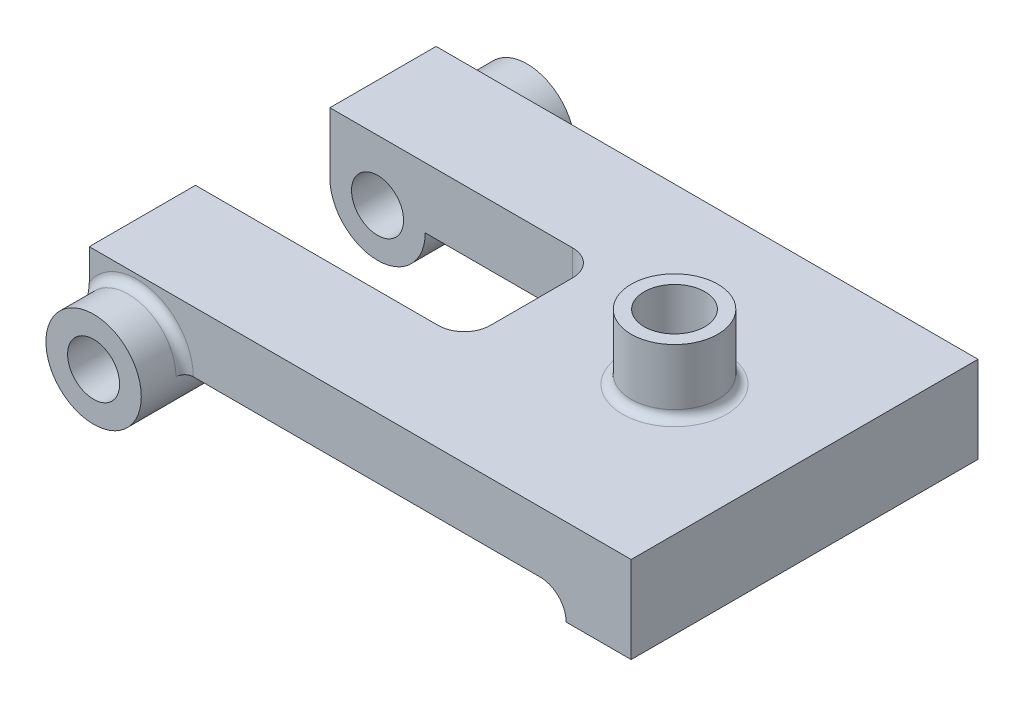
ISO-10303-21;
HEADER;
FILE_DESCRIPTION(('STEP AP214'),'2;1');
FILE_NAME('part.step','',(''),(''),'','','');
FILE_SCHEMA(('AUTOMOTIVE_DESIGN { 1 0 10303 214 1 1 1 1 }'));
ENDSEC;
DATA;
#1=APPLICATION_CONTEXT('core data for automotive mechanical design processes');
#2=APPLICATION_PROTOCOL_DEFINITION('international standard','automotive_design',2000,#1);
#3=PRODUCT_CONTEXT('',#1,'mechanical');
#4=PRODUCT('Part','Part','',(#3));
#5=PRODUCT_RELATED_PRODUCT_CATEGORY('part','',(#4));
#6=PRODUCT_DEFINITION_FORMATION('','',#4);
#7=PRODUCT_DEFINITION_CONTEXT('part definition',#1,'design');
#8=PRODUCT_DEFINITION('design','',#6,#7);
#9=PRODUCT_DEFINITION_SHAPE('','',#8);
#10=(LENGTH_UNIT() NAMED_UNIT(*) SI_UNIT(.MILLI.,.METRE.));
#11=(NAMED_UNIT(*) PLANE_ANGLE_UNIT() SI_UNIT($,.RADIAN.));
#12=(NAMED_UNIT(*) SI_UNIT($,.STERADIAN.) SOLID_ANGLE_UNIT());
#13=UNCERTAINTY_MEASURE_WITH_UNIT(LENGTH_MEASURE(1.E-05),#10,'distance_accuracy_value','');
#14=(GEOMETRIC_REPRESENTATION_CONTEXT(3) GLOBAL_UNCERTAINTY_ASSIGNED_CONTEXT((#13)) GLOBAL_UNIT_ASSIGNED_CONTEXT((#10,
#11,#12)) REPRESENTATION_CONTEXT('',''));
#15=CARTESIAN_POINT('',(0.,0.,0.));
#16=DIRECTION('',(0.,0.,1.));
#17=DIRECTION('',(1.,0.,0.));
#18=AXIS2_PLACEMENT_3D('',#15,#16,#17);
#19=CARTESIAN_POINT('',(0.,0.,40.));
#20=DIRECTION('',(-1.,0.,0.));
#21=DIRECTION('',(0.,0.,1.));
#22=AXIS2_PLACEMENT_3D('',#19,#20,#21);
#23=PLANE('',#22);
#24=DIRECTION('',(0.,1.,0.));
#25=VECTOR('',#24,1.);
#26=CARTESIAN_POINT('',(0.,-91.,15.5));
#27=LINE('',#26,#25);
#28=CARTESIAN_POINT('',(0.,0.,15.5));
#29=VERTEX_POINT('',#28);
#30=CARTESIAN_POINT('',(0.,14.,15.5));
#31=VERTEX_POINT('',#30);
#32=EDGE_CURVE('E184',#29,#31,#27,.T.);
#33=ORIENTED_EDGE('',*,*,#32,.F.);
#34=DIRECTION('',(0.,0.,-1.));
#35=VECTOR('',#34,1.);
#36=CARTESIAN_POINT('',(0.,0.,40.));
#37=LINE('',#36,#35);
#38=CARTESIAN_POINT('',(0.,0.,42.));
#39=VERTEX_POINT('',#38);
#40=EDGE_CURVE('E265',#39,#29,#37,.T.);
#41=ORIENTED_EDGE('',*,*,#40,.F.);
#42=CARTESIAN_POINT('',(0.,6.92820323027551,40.));
#43=CARTESIAN_POINT('',(0.,6.79631878338538,40.0000195877206));
#44=CARTESIAN_POINT('',(0.,6.6644773142545,40.0037039568171));
#45=CARTESIAN_POINT('',(0.,6.40121335984525,40.0176384033789));
#46=CARTESIAN_POINT('',(0.,6.26979067374991,40.0278846179913));
#47=CARTESIAN_POINT('',(0.,6.00790763005172,40.0541440086299));
#48=CARTESIAN_POINT('',(0.,5.8774456101869,40.0701410055856));
#49=CARTESIAN_POINT('',(0.,5.61724352656619,40.1072767015453));
#50=CARTESIAN_POINT('',(0.,5.48750358375657,40.1284162368858));
#51=CARTESIAN_POINT('',(0.,5.10222369832927,40.1981930126899));
#52=CARTESIAN_POINT('',(0.,4.84787990643271,40.2534888297203));
#53=CARTESIAN_POINT('',(0.,4.34256909228623,40.3782545428354));
#54=CARTESIAN_POINT('',(0.,4.09160501060128,40.4477360266855));
#55=CARTESIAN_POINT('',(0.,3.51579220612537,40.6210301613932));
#56=CARTESIAN_POINT('',(0.,3.1921467958774,40.7288093836496));
#57=CARTESIAN_POINT('',(0.,2.54957173398162,40.9576910405927));
#58=CARTESIAN_POINT('',(0.,2.23064375632872,41.0787980818546));
#59=CARTESIAN_POINT('',(0.,1.27744390124962,41.455368919855));
#60=CARTESIAN_POINT('',(0.,0.648288026431028,41.7235697880645));
#61=CARTESIAN_POINT('',(0.,0.0128635078759241,41.9945149951131));
#62=CARTESIAN_POINT('',(0.,0.00643174896304407,41.9972575065247));
#63=CARTESIAN_POINT('',(0.,0.,42.));
#64=B_SPLINE_CURVE_WITH_KNOTS('',3,(#42,#43,#44,#45,#46,#47,#48,#49,#50,#51,#52,#53,#54,#55,#56,
#57,#58,#59,#60,#61,#62,#63),.UNSPECIFIED.,.F.,.F.,(4,2,2,2,2,2,2,2,2,2,4),(0.,
0.395540642762623,0.790848650888232,1.18505310551169,1.57932171293576,2.35959856433425,
3.14051536472973,4.16341984179192,5.1866789886057,7.23803512077281,7.25901129773622),.UNSPECIFIED.);
#65=CARTESIAN_POINT('',(0.,6.92820323027551,40.));
#66=VERTEX_POINT('',#65);
#67=EDGE_CURVE('E278',#39,#66,#64,.F.);
#68=ORIENTED_EDGE('',*,*,#67,.T.);
#69=DIRECTION('',(0.,1.,0.));
#70=VECTOR('',#69,1.);
#71=CARTESIAN_POINT('',(0.,0.,40.));
#72=LINE('',#71,#70);
#73=CARTESIAN_POINT('',(0.,14.,40.));
#74=VERTEX_POINT('',#73);
#75=EDGE_CURVE('E231',#66,#74,#72,.T.);
#76=ORIENTED_EDGE('',*,*,#75,.T.);
#77=DIRECTION('',(0.,0.,-1.));
#78=VECTOR('',#77,1.);
#79=CARTESIAN_POINT('',(0.,14.,40.));
#80=LINE('',#79,#78);
#81=EDGE_CURVE('E270',#74,#31,#80,.T.);
#82=ORIENTED_EDGE('',*,*,#81,.T.);
#83=EDGE_LOOP('',(#33,#41,#68,#76,#82));
#84=FACE_BOUND('',#83,.T.);
#85=ADVANCED_FACE('F41',(#84),#23,.T.);
#86=CARTESIAN_POINT('',(11.,0.,50.));
#87=DIRECTION('',(0.,0.,-1.));
#88=DIRECTION('',(-1.,0.,0.));
#89=AXIS2_PLACEMENT_3D('',#86,#87,#88);
#90=CYLINDRICAL_SURFACE('',#89,6.);
#91=CARTESIAN_POINT('',(11.,0.,15.5));
#92=DIRECTION('',(0.,0.,1.));
#93=DIRECTION('',(1.,0.,0.));
#94=AXIS2_PLACEMENT_3D('',#91,#92,#93);
#95=CIRCLE('',#94,6.);
#96=CARTESIAN_POINT('',(5.,0.,15.5));
#97=VERTEX_POINT('',#96);
#98=EDGE_CURVE('E199',#97,#97,#95,.T.);
#99=CARTESIAN_POINT('',(11.,0.,50.));
#100=DIRECTION('',(0.,0.,1.));
#101=DIRECTION('',(1.,0.,0.));
#102=AXIS2_PLACEMENT_3D('',#99,#100,#101);
#103=CIRCLE('',#102,6.);
#104=CARTESIAN_POINT('',(5.,0.,50.));
#105=VERTEX_POINT('',#104);
#106=EDGE_CURVE('E206',#105,#105,#103,.T.);
#107=CARTESIAN_POINT('',(5.,0.,15.5));
#108=CARTESIAN_POINT('',(5.,0.,15.859375));
#109=CARTESIAN_POINT('',(5.,0.,16.21875));
#110=CARTESIAN_POINT('',(5.,0.,16.9375));
#111=CARTESIAN_POINT('',(5.,0.,17.296875));
#112=CARTESIAN_POINT('',(5.,0.,18.015625));
#113=CARTESIAN_POINT('',(5.,0.,18.375));
#114=CARTESIAN_POINT('',(5.,0.,19.09375));
#115=CARTESIAN_POINT('',(5.,0.,19.453125));
#116=CARTESIAN_POINT('',(5.,0.,20.171875));
#117=CARTESIAN_POINT('',(5.,0.,20.53125));
#118=CARTESIAN_POINT('',(5.,0.,21.25));
#119=CARTESIAN_POINT('',(5.,0.,21.609375));
#120=CARTESIAN_POINT('',(5.,0.,22.328125));
#121=CARTESIAN_POINT('',(5.,0.,22.6875));
#122=CARTESIAN_POINT('',(5.,0.,23.40625));
#123=CARTESIAN_POINT('',(5.,0.,23.765625));
#124=CARTESIAN_POINT('',(5.,0.,24.484375));
#125=CARTESIAN_POINT('',(5.,0.,24.84375));
#126=CARTESIAN_POINT('',(5.,0.,25.5625));
#127=CARTESIAN_POINT('',(5.,0.,25.921875));
#128=CARTESIAN_POINT('',(5.,0.,26.640625));
#129=CARTESIAN_POINT('',(5.,0.,27.));
#130=CARTESIAN_POINT('',(5.,0.,27.71875));
#131=CARTESIAN_POINT('',(5.,0.,28.078125));
#132=CARTESIAN_POINT('',(5.,0.,28.796875));
#133=CARTESIAN_POINT('',(5.,0.,29.15625));
#134=CARTESIAN_POINT('',(5.,0.,29.875));
#135=CARTESIAN_POINT('',(5.,0.,30.234375));
#136=CARTESIAN_POINT('',(5.,0.,30.953125));
#137=CARTESIAN_POINT('',(5.,0.,31.3125));
#138=CARTESIAN_POINT('',(5.,0.,32.03125));
#139=CARTESIAN_POINT('',(5.,0.,32.390625));
#140=CARTESIAN_POINT('',(5.,0.,33.109375));
#141=CARTESIAN_POINT('',(5.,0.,33.46875));
#142=CARTESIAN_POINT('',(5.,0.,34.1875));
#143=CARTESIAN_POINT('',(5.,0.,34.546875));
#144=CARTESIAN_POINT('',(5.,0.,35.265625));
#145=CARTESIAN_POINT('',(5.,0.,35.625));
#146=CARTESIAN_POINT('',(5.,0.,36.34375));
#147=CARTESIAN_POINT('',(5.,0.,36.703125));
#148=CARTESIAN_POINT('',(5.,0.,37.421875));
#149=CARTESIAN_POINT('',(5.,0.,37.78125));
#150=CARTESIAN_POINT('',(5.,0.,38.5));
#151=CARTESIAN_POINT('',(5.,0.,38.859375));
#152=CARTESIAN_POINT('',(5.,0.,39.578125));
#153=CARTESIAN_POINT('',(5.,0.,39.9375));
#154=CARTESIAN_POINT('',(5.,0.,40.65625));
#155=CARTESIAN_POINT('',(5.,0.,41.015625));
#156=CARTESIAN_POINT('',(5.,0.,41.734375));
#157=CARTESIAN_POINT('',(5.,0.,42.09375));
#158=CARTESIAN_POINT('',(5.,0.,42.8125));
#159=CARTESIAN_POINT('',(5.,0.,43.171875));
#160=CARTESIAN_POINT('',(5.,0.,43.890625));
#161=CARTESIAN_POINT('',(5.,0.,44.25));
#162=CARTESIAN_POINT('',(5.,0.,44.96875));
#163=CARTESIAN_POINT('',(5.,0.,45.328125));
#164=CARTESIAN_POINT('',(5.,0.,46.046875));
#165=CARTESIAN_POINT('',(5.,0.,46.40625));
#166=CARTESIAN_POINT('',(5.,0.,47.125));
#167=CARTESIAN_POINT('',(5.,0.,47.484375));
#168=CARTESIAN_POINT('',(5.,0.,48.203125));
#169=CARTESIAN_POINT('',(5.,0.,48.5625));
#170=CARTESIAN_POINT('',(5.,0.,49.28125));
#171=CARTESIAN_POINT('',(5.,0.,49.640625));
#172=CARTESIAN_POINT('',(5.,0.,50.));
#173=B_SPLINE_CURVE_WITH_KNOTS('',3,(#107,#108,#109,#110,#111,#112,#113,#114,#115,#116,#117,
#118,#119,#120,#121,#122,#123,#124,#125,#126,#127,#128,#129,#130,#131,#132,#133,#134,#135,#136,
#137,#138,#139,#140,#141,#142,#143,#144,#145,#146,#147,#148,#149,#150,#151,#152,#153,#154,#155,
#156,#157,#158,#159,#160,#161,#162,#163,#164,#165,#166,#167,#168,#169,#170,#171,#172),
.UNSPECIFIED.,.F.,.F.,(4,2,2,2,2,2,2,2,2,2,2,2,2,2,2,2,2,2,2,2,2,2,2,2,2,2,2,2,2,2,2,2,4),(0.,
1.078125,2.15625,3.234375,4.31249999999999,5.39062499999999,6.46874999999999,7.54687499999999,
8.62499999999999,9.70312499999999,10.78125,11.859375,12.9375,14.015625,15.09375,16.171875,17.25,
18.328125,19.40625,20.484375,21.5625,22.640625,23.71875,24.796875,25.875,26.953125,28.03125,
29.109375,30.1875,31.265625,32.34375,33.421875,34.5),.UNSPECIFIED.);
#174=EDGE_CURVE('BSEAM325',#97,#105,#173,.T.);
#175=ORIENTED_EDGE('',*,*,#98,.F.);
#176=ORIENTED_EDGE('',*,*,#106,.T.);
#177=ORIENTED_EDGE('',*,*,#174,.T.);
#178=ORIENTED_EDGE('',*,*,#174,.F.);
#179=EDGE_LOOP('',(#175,#177,#176,#178));
#180=FACE_BOUND('',#179,.T.);
#181=ADVANCED_FACE('F325',(#180),#90,.F.);
#182=CARTESIAN_POINT('',(11.,0.,50.));
#183=DIRECTION('',(0.,0.,-1.));
#184=DIRECTION('',(-1.,0.,0.));
#185=AXIS2_PLACEMENT_3D('',#182,#183,#184);
#186=CYLINDRICAL_SURFACE('',#185,11.);
#187=CARTESIAN_POINT('',(11.,0.,50.));
#188=DIRECTION('',(0.,0.,1.));
#189=DIRECTION('',(1.,0.,0.));
#190=AXIS2_PLACEMENT_3D('',#187,#188,#189);
#191=CIRCLE('',#190,11.);
#192=CARTESIAN_POINT('',(22.,0.,50.));
#193=VERTEX_POINT('',#192);
#194=EDGE_CURVE('E212',#193,#193,#191,.T.);
#195=ORIENTED_EDGE('',*,*,#194,.F.);
#196=EDGE_LOOP('',(#195));
#197=FACE_BOUND('',#196,.T.);
#198=ORIENTED_EDGE('',*,*,#40,.T.);
#199=CARTESIAN_POINT('',(11.,0.,15.5));
#200=DIRECTION('',(0.,0.,1.));
#201=DIRECTION('',(1.,0.,0.));
#202=AXIS2_PLACEMENT_3D('',#199,#200,#201);
#203=CIRCLE('',#202,11.);
#204=CARTESIAN_POINT('',(22.,0.,15.5));
#205=VERTEX_POINT('',#204);
#206=EDGE_CURVE('E340',#29,#205,#203,.T.);
#207=ORIENTED_EDGE('',*,*,#206,.T.);
#208=DIRECTION('',(0.,0.,-1.));
#209=VECTOR('',#208,1.);
#210=CARTESIAN_POINT('',(22.,0.,40.));
#211=LINE('',#210,#209);
#212=CARTESIAN_POINT('',(22.,0.,42.));
#213=VERTEX_POINT('',#212);
#214=EDGE_CURVE('E256',#213,#205,#211,.T.);
#215=ORIENTED_EDGE('',*,*,#214,.F.);
#216=CARTESIAN_POINT('',(11.,0.,42.));
#217=DIRECTION('',(0.,0.,1.));
#218=DIRECTION('',(1.,0.,0.));
#219=AXIS2_PLACEMENT_3D('',#216,#217,#218);
#220=CIRCLE('',#219,11.);
#221=EDGE_CURVE('E277',#213,#39,#220,.T.);
#222=ORIENTED_EDGE('',*,*,#221,.T.);
#223=EDGE_LOOP('',(#198,#207,#215,#222));
#224=FACE_BOUND('',#223,.T.);
#225=ADVANCED_FACE('F302',(#197,#224),#186,.T.);
#226=CARTESIAN_POINT('',(104.,-6.,40.));
#227=DIRECTION('',(0.,0.,-1.));
#228=DIRECTION('',(-1.,0.,0.));
#229=AXIS2_PLACEMENT_3D('',#226,#227,#228);
#230=CYLINDRICAL_SURFACE('',#229,6.);
#231=CARTESIAN_POINT('',(104.,-6.,-40.));
#232=DIRECTION('',(0.,0.,1.));
#233=DIRECTION('',(1.,0.,0.));
#234=AXIS2_PLACEMENT_3D('',#231,#232,#233);
#235=CIRCLE('',#234,6.);
#236=CARTESIAN_POINT('',(110.,-6.,-40.));
#237=VERTEX_POINT('',#236);
#238=CARTESIAN_POINT('',(104.,0.,-40.));
#239=VERTEX_POINT('',#238);
#240=EDGE_CURVE('E213',#237,#239,#235,.T.);
#241=ORIENTED_EDGE('',*,*,#240,.F.);
#242=DIRECTION('',(0.,0.,-1.));
#243=VECTOR('',#242,1.);
#244=CARTESIAN_POINT('',(110.,-6.,40.));
#245=LINE('',#244,#243);
#246=CARTESIAN_POINT('',(110.,-6.,40.));
#247=VERTEX_POINT('',#246);
#248=EDGE_CURVE('E274',#247,#237,#245,.T.);
#249=ORIENTED_EDGE('',*,*,#248,.F.);
#250=CARTESIAN_POINT('',(104.,-6.,40.));
#251=DIRECTION('',(0.,0.,1.));
#252=DIRECTION('',(1.,0.,0.));
#253=AXIS2_PLACEMENT_3D('',#250,#251,#252);
#254=CIRCLE('',#253,6.);
#255=CARTESIAN_POINT('',(104.,0.,40.));
#256=VERTEX_POINT('',#255);
#257=EDGE_CURVE('E218',#247,#256,#254,.T.);
#258=ORIENTED_EDGE('',*,*,#257,.T.);
#259=DIRECTION('',(0.,0.,-1.));
#260=VECTOR('',#259,1.);
#261=CARTESIAN_POINT('',(104.,0.,40.));
#262=LINE('',#261,#260);
#263=EDGE_CURVE('E240',#256,#239,#262,.T.);
#264=ORIENTED_EDGE('',*,*,#263,.T.);
#265=EDGE_LOOP('',(#241,#249,#258,#264));
#266=FACE_BOUND('',#265,.T.);
#267=ADVANCED_FACE('F297',(#266),#230,.F.);
#268=CARTESIAN_POINT('',(0.,-6.00000000000002,40.));
#269=DIRECTION('',(0.,-1.,0.));
#270=DIRECTION('',(1.,0.,0.));
#271=AXIS2_PLACEMENT_3D('',#268,#269,#270);
#272=PLANE('',#271);
#273=DIRECTION('',(-1.,0.,0.));
#274=VECTOR('',#273,1.);
#275=CARTESIAN_POINT('',(0.,-6.00000000000002,-40.));
#276=LINE('',#275,#274);
#277=CARTESIAN_POINT('',(125.,-6.,-40.));
#278=VERTEX_POINT('',#277);
#279=EDGE_CURVE('E239',#278,#237,#276,.T.);
#280=ORIENTED_EDGE('',*,*,#279,.F.);
#281=DIRECTION('',(0.,0.,-1.));
#282=VECTOR('',#281,1.);
#283=CARTESIAN_POINT('',(125.,-6.,40.));
#284=LINE('',#283,#282);
#285=CARTESIAN_POINT('',(125.,-6.,40.));
#286=VERTEX_POINT('',#285);
#287=EDGE_CURVE('E275',#286,#278,#284,.T.);
#288=ORIENTED_EDGE('',*,*,#287,.F.);
#289=DIRECTION('',(-1.,0.,0.));
#290=VECTOR('',#289,1.);
#291=CARTESIAN_POINT('',(0.,-6.00000000000002,40.));
#292=LINE('',#291,#290);
#293=EDGE_CURVE('E221',#286,#247,#292,.T.);
#294=ORIENTED_EDGE('',*,*,#293,.T.);
#295=ORIENTED_EDGE('',*,*,#248,.T.);
#296=EDGE_LOOP('',(#280,#288,#294,#295));
#297=FACE_BOUND('',#296,.T.);
#298=ADVANCED_FACE('F303',(#297),#272,.T.);
#299=CARTESIAN_POINT('',(125.,0.,40.));
#300=DIRECTION('',(1.,0.,0.));
#301=DIRECTION('',(0.,0.,-1.));
#302=AXIS2_PLACEMENT_3D('',#299,#300,#301);
#303=PLANE('',#302);
#304=DIRECTION('',(0.,-1.,0.));
#305=VECTOR('',#304,1.);
#306=CARTESIAN_POINT('',(125.,0.,-40.));
#307=LINE('',#306,#305);
#308=CARTESIAN_POINT('',(125.,14.,-40.));
#309=VERTEX_POINT('',#308);
#310=EDGE_CURVE('E243',#309,#278,#307,.T.);
#311=ORIENTED_EDGE('',*,*,#310,.F.);
#312=DIRECTION('',(0.,0.,-1.));
#313=VECTOR('',#312,1.);
#314=CARTESIAN_POINT('',(125.,14.,40.));
#315=LINE('',#314,#313);
#316=CARTESIAN_POINT('',(125.,14.,40.));
#317=VERTEX_POINT('',#316);
#318=EDGE_CURVE('E269',#317,#309,#315,.T.);
#319=ORIENTED_EDGE('',*,*,#318,.F.);
#320=DIRECTION('',(0.,-1.,0.));
#321=VECTOR('',#320,1.);
#322=CARTESIAN_POINT('',(125.,0.,40.));
#323=LINE('',#322,#321);
#324=EDGE_CURVE('E227',#317,#286,#323,.T.);
#325=ORIENTED_EDGE('',*,*,#324,.T.);
#326=ORIENTED_EDGE('',*,*,#287,.T.);
#327=EDGE_LOOP('',(#311,#319,#325,#326));
#328=FACE_BOUND('',#327,.T.);
#329=ADVANCED_FACE('F308',(#328),#303,.T.);
#330=CARTESIAN_POINT('',(0.,14.,40.));
#331=DIRECTION('',(0.,1.,0.));
#332=DIRECTION('',(0.,0.,1.));
#333=AXIS2_PLACEMENT_3D('',#330,#331,#332);
#334=PLANE('',#333);
#335=CARTESIAN_POINT('',(95.,14.,0.));
#336=DIRECTION('',(0.,1.,0.));
#337=DIRECTION('',(0.,0.,1.));
#338=AXIS2_PLACEMENT_3D('',#335,#336,#337);
#339=CIRCLE('',#338,12.);
#340=CARTESIAN_POINT('',(95.,14.,12.));
#341=VERTEX_POINT('',#340);
#342=EDGE_CURVE('E11',#341,#341,#339,.F.);
#343=ORIENTED_EDGE('',*,*,#342,.T.);
#344=EDGE_LOOP('',(#343));
#345=FACE_BOUND('',#344,.T.);
#346=DIRECTION('',(1.,0.,0.));
#347=VECTOR('',#346,1.);
#348=CARTESIAN_POINT('',(56.,14.,15.5));
#349=LINE('',#348,#347);
#350=CARTESIAN_POINT('',(56.,14.,15.5));
#351=VERTEX_POINT('',#350);
#352=EDGE_CURVE('E162',#31,#351,#349,.T.);
#353=ORIENTED_EDGE('',*,*,#352,.F.);
#354=ORIENTED_EDGE('',*,*,#81,.F.);
#355=DIRECTION('',(1.,0.,0.));
#356=VECTOR('',#355,1.);
#357=CARTESIAN_POINT('',(0.,14.,40.));
#358=LINE('',#357,#356);
#359=EDGE_CURVE('E229',#74,#317,#358,.T.);
#360=ORIENTED_EDGE('',*,*,#359,.T.);
#361=ORIENTED_EDGE('',*,*,#318,.T.);
#362=DIRECTION('',(1.,0.,0.));
#363=VECTOR('',#362,1.);
#364=CARTESIAN_POINT('',(0.,14.,-40.));
#365=LINE('',#364,#363);
#366=CARTESIAN_POINT('',(0.,14.,-40.));
#367=VERTEX_POINT('',#366);
#368=EDGE_CURVE('E246',#367,#309,#365,.T.);
#369=ORIENTED_EDGE('',*,*,#368,.F.);
#370=CARTESIAN_POINT('',(0.,14.,-15.5));
#371=VERTEX_POINT('',#370);
#372=EDGE_CURVE('E268',#371,#367,#80,.T.);
#373=ORIENTED_EDGE('',*,*,#372,.F.);
#374=DIRECTION('',(-1.,0.,0.));
#375=VECTOR('',#374,1.);
#376=CARTESIAN_POINT('',(0.,14.,-15.5));
#377=LINE('',#376,#375);
#378=CARTESIAN_POINT('',(56.,14.,-15.5));
#379=VERTEX_POINT('',#378);
#380=EDGE_CURVE('E178',#379,#371,#377,.T.);
#381=ORIENTED_EDGE('',*,*,#380,.F.);
#382=CARTESIAN_POINT('',(56.,14.,-9.5));
#383=DIRECTION('',(0.,1.,0.));
#384=DIRECTION('',(0.,0.,1.));
#385=AXIS2_PLACEMENT_3D('',#382,#383,#384);
#386=CIRCLE('',#385,6.);
#387=CARTESIAN_POINT('',(62.,14.,-9.49999999999996));
#388=VERTEX_POINT('',#387);
#389=EDGE_CURVE('E176',#388,#379,#386,.T.);
#390=ORIENTED_EDGE('',*,*,#389,.F.);
#391=DIRECTION('',(0.,0.,-1.));
#392=VECTOR('',#391,1.);
#393=CARTESIAN_POINT('',(62.,14.,-9.49999999999996));
#394=LINE('',#393,#392);
#395=CARTESIAN_POINT('',(62.,14.,9.49999999999996));
#396=VERTEX_POINT('',#395);
#397=EDGE_CURVE('E153',#396,#388,#394,.T.);
#398=ORIENTED_EDGE('',*,*,#397,.F.);
#399=CARTESIAN_POINT('',(56.,14.,9.5));
#400=DIRECTION('',(0.,1.,0.));
#401=DIRECTION('',(0.,0.,1.));
#402=AXIS2_PLACEMENT_3D('',#399,#400,#401);
#403=CIRCLE('',#402,6.);
#404=EDGE_CURVE('E164',#351,#396,#403,.T.);
#405=ORIENTED_EDGE('',*,*,#404,.F.);
#406=EDGE_LOOP('',(#353,#354,#360,#361,#369,#373,#381,#390,#398,#405));
#407=FACE_BOUND('',#406,.T.);
#408=ADVANCED_FACE('F173',(#345,#407),#334,.T.);
#409=DIRECTION('',(0.,1.,0.));
#410=VECTOR('',#409,1.);
#411=CARTESIAN_POINT('',(0.,-91.,-15.5));
#412=LINE('',#411,#410);
#413=CARTESIAN_POINT('',(0.,0.,-15.5));
#414=VERTEX_POINT('',#413);
#415=EDGE_CURVE('E57',#414,#371,#412,.T.);
#416=ORIENTED_EDGE('',*,*,#415,.T.);
#417=ORIENTED_EDGE('',*,*,#372,.T.);
#418=DIRECTION('',(0.,1.,0.));
#419=VECTOR('',#418,1.);
#420=CARTESIAN_POINT('',(0.,0.,-40.));
#421=LINE('',#420,#419);
#422=CARTESIAN_POINT('',(0.,0.,-40.));
#423=VERTEX_POINT('',#422);
#424=EDGE_CURVE('E248',#423,#367,#421,.T.);
#425=ORIENTED_EDGE('',*,*,#424,.F.);
#426=EDGE_CURVE('E264',#414,#423,#37,.T.);
#427=ORIENTED_EDGE('',*,*,#426,.F.);
#428=EDGE_LOOP('',(#416,#417,#425,#427));
#429=FACE_BOUND('',#428,.T.);
#430=ADVANCED_FACE('F287',(#429),#23,.T.);
#431=CARTESIAN_POINT('',(0.,0.,40.));
#432=DIRECTION('',(0.,-1.,0.));
#433=DIRECTION('',(1.,0.,0.));
#434=AXIS2_PLACEMENT_3D('',#431,#432,#433);
#435=PLANE('',#434);
#436=DIRECTION('',(-1.,0.,0.));
#437=VECTOR('',#436,1.);
#438=CARTESIAN_POINT('',(0.,0.,15.5));
#439=LINE('',#438,#437);
#440=CARTESIAN_POINT('',(56.,0.,15.5));
#441=VERTEX_POINT('',#440);
#442=EDGE_CURVE('E193',#441,#205,#439,.T.);
#443=ORIENTED_EDGE('',*,*,#442,.F.);
#444=CARTESIAN_POINT('',(56.,0.,9.5));
#445=DIRECTION('',(0.,-1.,0.));
#446=DIRECTION('',(1.,0.,0.));
#447=AXIS2_PLACEMENT_3D('',#444,#445,#446);
#448=CIRCLE('',#447,6.);
#449=CARTESIAN_POINT('',(62.,0.,9.49999999999996));
#450=VERTEX_POINT('',#449);
#451=EDGE_CURVE('E353',#450,#441,#448,.T.);
#452=ORIENTED_EDGE('',*,*,#451,.F.);
#453=DIRECTION('',(0.,0.,1.));
#454=VECTOR('',#453,1.);
#455=CARTESIAN_POINT('',(62.,0.,40.));
#456=LINE('',#455,#454);
#457=CARTESIAN_POINT('',(62.,0.,-9.49999999999996));
#458=VERTEX_POINT('',#457);
#459=EDGE_CURVE('E156',#458,#450,#456,.T.);
#460=ORIENTED_EDGE('',*,*,#459,.F.);
#461=CARTESIAN_POINT('',(56.,0.,-9.5));
#462=DIRECTION('',(0.,-1.,0.));
#463=DIRECTION('',(1.,0.,0.));
#464=AXIS2_PLACEMENT_3D('',#461,#462,#463);
#465=CIRCLE('',#464,6.);
#466=CARTESIAN_POINT('',(56.,0.,-15.5));
#467=VERTEX_POINT('',#466);
#468=EDGE_CURVE('E359',#467,#458,#465,.T.);
#469=ORIENTED_EDGE('',*,*,#468,.F.);
#470=DIRECTION('',(1.,0.,0.));
#471=VECTOR('',#470,1.);
#472=CARTESIAN_POINT('',(0.,0.,-15.5));
#473=LINE('',#472,#471);
#474=CARTESIAN_POINT('',(22.,0.,-15.5));
#475=VERTEX_POINT('',#474);
#476=EDGE_CURVE('E183',#475,#467,#473,.T.);
#477=ORIENTED_EDGE('',*,*,#476,.F.);
#478=CARTESIAN_POINT('',(22.,0.,-40.));
#479=VERTEX_POINT('',#478);
#480=EDGE_CURVE('E259',#475,#479,#211,.T.);
#481=ORIENTED_EDGE('',*,*,#480,.T.);
#482=DIRECTION('',(-1.,0.,0.));
#483=VECTOR('',#482,1.);
#484=CARTESIAN_POINT('',(0.,0.,-40.));
#485=LINE('',#484,#483);
#486=EDGE_CURVE('E222',#239,#479,#485,.T.);
#487=ORIENTED_EDGE('',*,*,#486,.F.);
#488=ORIENTED_EDGE('',*,*,#263,.F.);
#489=DIRECTION('',(-1.,0.,0.));
#490=VECTOR('',#489,1.);
#491=CARTESIAN_POINT('',(0.,0.,40.));
#492=LINE('',#491,#490);
#493=CARTESIAN_POINT('',(24.,0.,40.));
#494=VERTEX_POINT('',#493);
#495=EDGE_CURVE('E232',#256,#494,#492,.T.);
#496=ORIENTED_EDGE('',*,*,#495,.T.);
#497=CARTESIAN_POINT('',(24.,0.,42.));
#498=DIRECTION('',(0.,-1.,0.));
#499=DIRECTION('',(1.,0.,0.));
#500=AXIS2_PLACEMENT_3D('',#497,#498,#499);
#501=CIRCLE('',#500,2.);
#502=EDGE_CURVE('E290',#494,#213,#501,.F.);
#503=ORIENTED_EDGE('',*,*,#502,.T.);
#504=ORIENTED_EDGE('',*,*,#214,.T.);
#505=EDGE_LOOP('',(#443,#452,#460,#469,#477,#481,#487,#488,#496,#503,#504));
#506=FACE_BOUND('',#505,.T.);
#507=CARTESIAN_POINT('',(95.,0.,0.));
#508=DIRECTION('',(0.,-1.,0.));
#509=DIRECTION('',(1.,0.,0.));
#510=AXIS2_PLACEMENT_3D('',#507,#508,#509);
#511=CIRCLE('',#510,7.);
#512=CARTESIAN_POINT('',(102.,0.,0.));
#513=VERTEX_POINT('',#512);
#514=EDGE_CURVE('E198',#513,#513,#511,.T.);
#515=ORIENTED_EDGE('',*,*,#514,.F.);
#516=EDGE_LOOP('',(#515));
#517=FACE_BOUND('',#516,.T.);
#518=ADVANCED_FACE('F316',(#506,#517),#435,.T.);
#519=CARTESIAN_POINT('',(0.,0.,40.));
#520=DIRECTION('',(0.,0.,1.));
#521=DIRECTION('',(1.,0.,0.));
#522=AXIS2_PLACEMENT_3D('',#519,#520,#521);
#523=PLANE('',#522);
#524=ORIENTED_EDGE('',*,*,#75,.F.);
#525=CARTESIAN_POINT('',(11.,0.,40.));
#526=DIRECTION('',(0.,0.,1.));
#527=DIRECTION('',(1.,0.,0.));
#528=AXIS2_PLACEMENT_3D('',#525,#526,#527);
#529=CIRCLE('',#528,13.);
#530=EDGE_CURVE('E61',#66,#494,#529,.F.);
#531=ORIENTED_EDGE('',*,*,#530,.T.);
#532=ORIENTED_EDGE('',*,*,#495,.F.);
#533=ORIENTED_EDGE('',*,*,#257,.F.);
#534=ORIENTED_EDGE('',*,*,#293,.F.);
#535=ORIENTED_EDGE('',*,*,#324,.F.);
#536=ORIENTED_EDGE('',*,*,#359,.F.);
#537=EDGE_LOOP('',(#524,#531,#532,#533,#534,#535,#536));
#538=FACE_BOUND('',#537,.T.);
#539=ADVANCED_FACE('F345',(#538),#523,.T.);
#540=CARTESIAN_POINT('',(0.,0.,-40.));
#541=DIRECTION('',(0.,0.,1.));
#542=DIRECTION('',(1.,0.,0.));
#543=AXIS2_PLACEMENT_3D('',#540,#541,#542);
#544=PLANE('',#543);
#545=ORIENTED_EDGE('',*,*,#240,.T.);
#546=ORIENTED_EDGE('',*,*,#486,.T.);
#547=CARTESIAN_POINT('',(11.,0.,-40.));
#548=DIRECTION('',(0.,0.,1.));
#549=DIRECTION('',(1.,0.,0.));
#550=AXIS2_PLACEMENT_3D('',#547,#548,#549);
#551=CIRCLE('',#550,11.);
#552=EDGE_CURVE('E255',#479,#423,#551,.T.);
#553=ORIENTED_EDGE('',*,*,#552,.T.);
#554=ORIENTED_EDGE('',*,*,#424,.T.);
#555=ORIENTED_EDGE('',*,*,#368,.T.);
#556=ORIENTED_EDGE('',*,*,#310,.T.);
#557=ORIENTED_EDGE('',*,*,#279,.T.);
#558=EDGE_LOOP('',(#545,#546,#553,#554,#555,#556,#557));
#559=FACE_BOUND('',#558,.T.);
#560=ADVANCED_FACE('F401',(#559),#544,.F.);
#561=CARTESIAN_POINT('',(11.,0.,-15.5));
#562=DIRECTION('',(0.,0.,-1.));
#563=DIRECTION('',(-1.,0.,0.));
#564=AXIS2_PLACEMENT_3D('',#561,#562,#563);
#565=CIRCLE('',#564,6.);
#566=CARTESIAN_POINT('',(5.,0.,-15.5));
#567=VERTEX_POINT('',#566);
#568=EDGE_CURVE('E195',#567,#567,#565,.T.);
#569=CARTESIAN_POINT('',(11.,0.,-50.));
#570=DIRECTION('',(0.,0.,1.));
#571=DIRECTION('',(1.,0.,0.));
#572=AXIS2_PLACEMENT_3D('',#569,#570,#571);
#573=CIRCLE('',#572,6.);
#574=CARTESIAN_POINT('',(5.,0.,-50.));
#575=VERTEX_POINT('',#574);
#576=EDGE_CURVE('E210',#575,#575,#573,.T.);
#577=CARTESIAN_POINT('',(5.,0.,-15.5));
#578=CARTESIAN_POINT('',(5.,0.,-15.859375));
#579=CARTESIAN_POINT('',(5.,0.,-16.21875));
#580=CARTESIAN_POINT('',(5.,0.,-16.9375));
#581=CARTESIAN_POINT('',(5.,0.,-17.296875));
#582=CARTESIAN_POINT('',(5.,0.,-18.015625));
#583=CARTESIAN_POINT('',(5.,0.,-18.375));
#584=CARTESIAN_POINT('',(5.,0.,-19.09375));
#585=CARTESIAN_POINT('',(5.,0.,-19.453125));
#586=CARTESIAN_POINT('',(5.,0.,-20.171875));
#587=CARTESIAN_POINT('',(5.,0.,-20.53125));
#588=CARTESIAN_POINT('',(5.,0.,-21.25));
#589=CARTESIAN_POINT('',(5.,0.,-21.609375));
#590=CARTESIAN_POINT('',(5.,0.,-22.328125));
#591=CARTESIAN_POINT('',(5.,0.,-22.6875));
#592=CARTESIAN_POINT('',(5.,0.,-23.40625));
#593=CARTESIAN_POINT('',(5.,0.,-23.765625));
#594=CARTESIAN_POINT('',(5.,0.,-24.484375));
#595=CARTESIAN_POINT('',(5.,0.,-24.84375));
#596=CARTESIAN_POINT('',(5.,0.,-25.5625));
#597=CARTESIAN_POINT('',(5.,0.,-25.921875));
#598=CARTESIAN_POINT('',(5.,0.,-26.640625));
#599=CARTESIAN_POINT('',(5.,0.,-27.));
#600=CARTESIAN_POINT('',(5.,0.,-27.71875));
#601=CARTESIAN_POINT('',(5.,0.,-28.078125));
#602=CARTESIAN_POINT('',(5.,0.,-28.796875));
#603=CARTESIAN_POINT('',(5.,0.,-29.15625));
#604=CARTESIAN_POINT('',(5.,0.,-29.875));
#605=CARTESIAN_POINT('',(5.,0.,-30.234375));
#606=CARTESIAN_POINT('',(5.,0.,-30.953125));
#607=CARTESIAN_POINT('',(5.,0.,-31.3125));
#608=CARTESIAN_POINT('',(5.,0.,-32.03125));
#609=CARTESIAN_POINT('',(5.,0.,-32.390625));
#610=CARTESIAN_POINT('',(5.,0.,-33.109375));
#611=CARTESIAN_POINT('',(5.,0.,-33.46875));
#612=CARTESIAN_POINT('',(5.,0.,-34.1875));
#613=CARTESIAN_POINT('',(5.,0.,-34.546875));
#614=CARTESIAN_POINT('',(5.,0.,-35.265625));
#615=CARTESIAN_POINT('',(5.,0.,-35.625));
#616=CARTESIAN_POINT('',(5.,0.,-36.34375));
#617=CARTESIAN_POINT('',(5.,0.,-36.703125));
#618=CARTESIAN_POINT('',(5.,0.,-37.421875));
#619=CARTESIAN_POINT('',(5.,0.,-37.78125));
#620=CARTESIAN_POINT('',(5.,0.,-38.5));
#621=CARTESIAN_POINT('',(5.,0.,-38.859375));
#622=CARTESIAN_POINT('',(5.,0.,-39.578125));
#623=CARTESIAN_POINT('',(5.,0.,-39.9375));
#624=CARTESIAN_POINT('',(5.,0.,-40.65625));
#625=CARTESIAN_POINT('',(5.,0.,-41.015625));
#626=CARTESIAN_POINT('',(5.,0.,-41.734375));
#627=CARTESIAN_POINT('',(5.,0.,-42.09375));
#628=CARTESIAN_POINT('',(5.,0.,-42.8125));
#629=CARTESIAN_POINT('',(5.,0.,-43.171875));
#630=CARTESIAN_POINT('',(5.,0.,-43.890625));
#631=CARTESIAN_POINT('',(5.,0.,-44.25));
#632=CARTESIAN_POINT('',(5.,0.,-44.96875));
#633=CARTESIAN_POINT('',(5.,0.,-45.328125));
#634=CARTESIAN_POINT('',(5.,0.,-46.046875));
#635=CARTESIAN_POINT('',(5.,0.,-46.40625));
#636=CARTESIAN_POINT('',(5.,0.,-47.125));
#637=CARTESIAN_POINT('',(5.,0.,-47.484375));
#638=CARTESIAN_POINT('',(5.,0.,-48.203125));
#639=CARTESIAN_POINT('',(5.,0.,-48.5625));
#640=CARTESIAN_POINT('',(5.,0.,-49.28125));
#641=CARTESIAN_POINT('',(5.,0.,-49.640625));
#642=CARTESIAN_POINT('',(5.,0.,-50.));
#643=B_SPLINE_CURVE_WITH_KNOTS('',3,(#577,#578,#579,#580,#581,#582,#583,#584,#585,#586,#587,
#588,#589,#590,#591,#592,#593,#594,#595,#596,#597,#598,#599,#600,#601,#602,#603,#604,#605,#606,
#607,#608,#609,#610,#611,#612,#613,#614,#615,#616,#617,#618,#619,#620,#621,#622,#623,#624,#625,
#626,#627,#628,#629,#630,#631,#632,#633,#634,#635,#636,#637,#638,#639,#640,#641,#642),
.UNSPECIFIED.,.F.,.F.,(4,2,2,2,2,2,2,2,2,2,2,2,2,2,2,2,2,2,2,2,2,2,2,2,2,2,2,2,2,2,2,2,4),(0.,
1.078125,2.15625,3.234375,4.3125,5.390625,6.46875,7.54687499999999,8.62499999999999,
9.70312500000001,10.78125,11.859375,12.9375,14.015625,15.09375,16.171875,17.25,18.328125,
19.40625,20.484375,21.5625,22.640625,23.71875,24.796875,25.875,26.953125,28.03125,29.109375,
30.1875,31.265625,32.34375,33.421875,34.5),.UNSPECIFIED.);
#644=EDGE_CURVE('BSEAM328',#567,#575,#643,.T.);
#645=ORIENTED_EDGE('',*,*,#568,.F.);
#646=ORIENTED_EDGE('',*,*,#576,.F.);
#647=ORIENTED_EDGE('',*,*,#644,.T.);
#648=ORIENTED_EDGE('',*,*,#644,.F.);
#649=EDGE_LOOP('',(#645,#647,#646,#648));
#650=FACE_BOUND('',#649,.T.);
#651=ADVANCED_FACE('F328',(#650),#90,.F.);
#652=ORIENTED_EDGE('',*,*,#480,.F.);
#653=CARTESIAN_POINT('',(11.,0.,-15.5));
#654=DIRECTION('',(0.,0.,-1.));
#655=DIRECTION('',(-1.,0.,0.));
#656=AXIS2_PLACEMENT_3D('',#653,#654,#655);
#657=CIRCLE('',#656,11.);
#658=EDGE_CURVE('E355',#475,#414,#657,.T.);
#659=ORIENTED_EDGE('',*,*,#658,.T.);
#660=ORIENTED_EDGE('',*,*,#426,.T.);
#661=ORIENTED_EDGE('',*,*,#552,.F.);
#662=EDGE_LOOP('',(#652,#659,#660,#661));
#663=FACE_BOUND('',#662,.T.);
#664=CARTESIAN_POINT('',(11.,0.,-50.));
#665=DIRECTION('',(0.,0.,1.));
#666=DIRECTION('',(1.,0.,0.));
#667=AXIS2_PLACEMENT_3D('',#664,#665,#666);
#668=CIRCLE('',#667,11.);
#669=CARTESIAN_POINT('',(22.,0.,-50.));
#670=VERTEX_POINT('',#669);
#671=EDGE_CURVE('E215',#670,#670,#668,.T.);
#672=ORIENTED_EDGE('',*,*,#671,.T.);
#673=EDGE_LOOP('',(#672));
#674=FACE_BOUND('',#673,.T.);
#675=ADVANCED_FACE('F393',(#663,#674),#186,.T.);
#676=CARTESIAN_POINT('',(0.,0.,50.));
#677=DIRECTION('',(0.,0.,1.));
#678=DIRECTION('',(1.,0.,0.));
#679=AXIS2_PLACEMENT_3D('',#676,#677,#678);
#680=PLANE('',#679);
#681=ORIENTED_EDGE('',*,*,#106,.F.);
#682=EDGE_LOOP('',(#681));
#683=FACE_BOUND('',#682,.T.);
#684=ORIENTED_EDGE('',*,*,#194,.T.);
#685=EDGE_LOOP('',(#684));
#686=FACE_BOUND('',#685,.T.);
#687=ADVANCED_FACE('F394',(#683,#686),#680,.T.);
#688=CARTESIAN_POINT('',(0.,0.,-50.));
#689=DIRECTION('',(0.,0.,1.));
#690=DIRECTION('',(1.,0.,0.));
#691=AXIS2_PLACEMENT_3D('',#688,#689,#690);
#692=PLANE('',#691);
#693=ORIENTED_EDGE('',*,*,#576,.T.);
#694=EDGE_LOOP('',(#693));
#695=FACE_BOUND('',#694,.T.);
#696=ORIENTED_EDGE('',*,*,#671,.F.);
#697=EDGE_LOOP('',(#696));
#698=FACE_BOUND('',#697,.T.);
#699=ADVANCED_FACE('F296',(#695,#698),#692,.F.);
#700=CARTESIAN_POINT('',(11.,0.,42.));
#701=DIRECTION('',(0.,0.,1.));
#702=DIRECTION('',(1.,0.,0.));
#703=AXIS2_PLACEMENT_3D('',#700,#701,#702);
#704=TOROIDAL_SURFACE('',#703,13.,2.);
#705=ORIENTED_EDGE('',*,*,#502,.F.);
#706=ORIENTED_EDGE('',*,*,#530,.F.);
#707=ORIENTED_EDGE('',*,*,#67,.F.);
#708=ORIENTED_EDGE('',*,*,#221,.F.);
#709=EDGE_LOOP('',(#705,#706,#707,#708));
#710=FACE_BOUND('',#709,.T.);
#711=ADVANCED_FACE('F291',(#710),#704,.F.);
#712=CARTESIAN_POINT('',(95.,29.,0.));
#713=DIRECTION('',(0.,1.,0.));
#714=DIRECTION('',(0.,0.,1.));
#715=AXIS2_PLACEMENT_3D('',#712,#713,#714);
#716=PLANE('',#715);
#717=CARTESIAN_POINT('',(95.,29.,0.));
#718=DIRECTION('',(0.,1.,0.));
#719=DIRECTION('',(0.,0.,1.));
#720=AXIS2_PLACEMENT_3D('',#717,#718,#719);
#721=CIRCLE('',#720,9.99999999999999);
#722=CARTESIAN_POINT('',(95.,29.,9.99999999999999));
#723=VERTEX_POINT('',#722);
#724=EDGE_CURVE('E202',#723,#723,#721,.T.);
#725=ORIENTED_EDGE('',*,*,#724,.T.);
#726=EDGE_LOOP('',(#725));
#727=FACE_BOUND('',#726,.T.);
#728=CARTESIAN_POINT('',(95.,29.,0.));
#729=DIRECTION('',(0.,1.,0.));
#730=DIRECTION('',(0.,0.,1.));
#731=AXIS2_PLACEMENT_3D('',#728,#729,#730);
#732=CIRCLE('',#731,7.);
#733=CARTESIAN_POINT('',(95.,29.,7.));
#734=VERTEX_POINT('',#733);
#735=EDGE_CURVE('E203',#734,#734,#732,.T.);
#736=ORIENTED_EDGE('',*,*,#735,.F.);
#737=EDGE_LOOP('',(#736));
#738=FACE_BOUND('',#737,.T.);
#739=ADVANCED_FACE('F300',(#727,#738),#716,.T.);
#740=CARTESIAN_POINT('',(95.,29.,0.));
#741=DIRECTION('',(0.,-1.,0.));
#742=DIRECTION('',(0.,0.,-1.));
#743=AXIS2_PLACEMENT_3D('',#740,#741,#742);
#744=CYLINDRICAL_SURFACE('',#743,9.99999999999999);
#745=CARTESIAN_POINT('',(95.,16.,0.));
#746=DIRECTION('',(0.,1.,0.));
#747=DIRECTION('',(0.,0.,1.));
#748=AXIS2_PLACEMENT_3D('',#745,#746,#747);
#749=CIRCLE('',#748,9.99999999999999);
#750=CARTESIAN_POINT('',(95.,16.,9.99999999999999));
#751=VERTEX_POINT('',#750);
#752=EDGE_CURVE('E47',#751,#751,#749,.T.);
#753=ORIENTED_EDGE('',*,*,#752,.T.);
#754=EDGE_LOOP('',(#753));
#755=FACE_BOUND('',#754,.T.);
#756=ORIENTED_EDGE('',*,*,#724,.F.);
#757=EDGE_LOOP('',(#756));
#758=FACE_BOUND('',#757,.T.);
#759=ADVANCED_FACE('F362',(#755,#758),#744,.T.);
#760=CARTESIAN_POINT('',(95.,29.,0.));
#761=DIRECTION('',(0.,-1.,0.));
#762=DIRECTION('',(0.,0.,-1.));
#763=AXIS2_PLACEMENT_3D('',#760,#761,#762);
#764=CYLINDRICAL_SURFACE('',#763,7.);
#765=ORIENTED_EDGE('',*,*,#735,.T.);
#766=EDGE_LOOP('',(#765));
#767=FACE_BOUND('',#766,.T.);
#768=ORIENTED_EDGE('',*,*,#514,.T.);
#769=EDGE_LOOP('',(#768));
#770=FACE_BOUND('',#769,.T.);
#771=ADVANCED_FACE('F383',(#767,#770),#764,.F.);
#772=CARTESIAN_POINT('',(56.,-91.,9.5));
#773=DIRECTION('',(0.,1.,0.));
#774=DIRECTION('',(0.,0.,1.));
#775=AXIS2_PLACEMENT_3D('',#772,#773,#774);
#776=CYLINDRICAL_SURFACE('',#775,6.);
#777=ORIENTED_EDGE('',*,*,#451,.T.);
#778=DIRECTION('',(0.,1.,0.));
#779=VECTOR('',#778,1.);
#780=CARTESIAN_POINT('',(56.,-91.,15.5));
#781=LINE('',#780,#779);
#782=EDGE_CURVE('E166',#441,#351,#781,.T.);
#783=ORIENTED_EDGE('',*,*,#782,.T.);
#784=ORIENTED_EDGE('',*,*,#404,.T.);
#785=DIRECTION('',(0.,1.,0.));
#786=VECTOR('',#785,1.);
#787=CARTESIAN_POINT('',(62.,-91.,9.49999999999996));
#788=LINE('',#787,#786);
#789=EDGE_CURVE('E148',#450,#396,#788,.T.);
#790=ORIENTED_EDGE('',*,*,#789,.F.);
#791=EDGE_LOOP('',(#777,#783,#784,#790));
#792=FACE_BOUND('',#791,.T.);
#793=ADVANCED_FACE('F168',(#792),#776,.F.);
#794=CARTESIAN_POINT('',(56.,-91.,15.5));
#795=DIRECTION('',(0.,0.,1.));
#796=DIRECTION('',(1.,0.,0.));
#797=AXIS2_PLACEMENT_3D('',#794,#795,#796);
#798=PLANE('',#797);
#799=ORIENTED_EDGE('',*,*,#98,.T.);
#800=EDGE_LOOP('',(#799));
#801=FACE_BOUND('',#800,.T.);
#802=ORIENTED_EDGE('',*,*,#442,.T.);
#803=ORIENTED_EDGE('',*,*,#206,.F.);
#804=ORIENTED_EDGE('',*,*,#32,.T.);
#805=ORIENTED_EDGE('',*,*,#352,.T.);
#806=ORIENTED_EDGE('',*,*,#782,.F.);
#807=EDGE_LOOP('',(#802,#803,#804,#805,#806));
#808=FACE_BOUND('',#807,.T.);
#809=ADVANCED_FACE('F349',(#801,#808),#798,.F.);
#810=CARTESIAN_POINT('',(0.,-91.,-15.5));
#811=DIRECTION('',(0.,0.,-1.));
#812=DIRECTION('',(-1.,0.,0.));
#813=AXIS2_PLACEMENT_3D('',#810,#811,#812);
#814=PLANE('',#813);
#815=ORIENTED_EDGE('',*,*,#568,.T.);
#816=EDGE_LOOP('',(#815));
#817=FACE_BOUND('',#816,.T.);
#818=ORIENTED_EDGE('',*,*,#476,.T.);
#819=DIRECTION('',(0.,1.,0.));
#820=VECTOR('',#819,1.);
#821=CARTESIAN_POINT('',(56.,-91.,-15.5));
#822=LINE('',#821,#820);
#823=EDGE_CURVE('E189',#467,#379,#822,.T.);
#824=ORIENTED_EDGE('',*,*,#823,.T.);
#825=ORIENTED_EDGE('',*,*,#380,.T.);
#826=ORIENTED_EDGE('',*,*,#415,.F.);
#827=ORIENTED_EDGE('',*,*,#658,.F.);
#828=EDGE_LOOP('',(#818,#824,#825,#826,#827));
#829=FACE_BOUND('',#828,.T.);
#830=ADVANCED_FACE('F377',(#817,#829),#814,.F.);
#831=CARTESIAN_POINT('',(56.,-91.,-9.5));
#832=DIRECTION('',(0.,1.,0.));
#833=DIRECTION('',(0.,0.,1.));
#834=AXIS2_PLACEMENT_3D('',#831,#832,#833);
#835=CYLINDRICAL_SURFACE('',#834,6.);
#836=ORIENTED_EDGE('',*,*,#468,.T.);
#837=DIRECTION('',(0.,1.,0.));
#838=VECTOR('',#837,1.);
#839=CARTESIAN_POINT('',(62.,-91.,-9.49999999999996));
#840=LINE('',#839,#838);
#841=EDGE_CURVE('E163',#458,#388,#840,.T.);
#842=ORIENTED_EDGE('',*,*,#841,.T.);
#843=ORIENTED_EDGE('',*,*,#389,.T.);
#844=ORIENTED_EDGE('',*,*,#823,.F.);
#845=EDGE_LOOP('',(#836,#842,#843,#844));
#846=FACE_BOUND('',#845,.T.);
#847=ADVANCED_FACE('F375',(#846),#835,.F.);
#848=CARTESIAN_POINT('',(62.,-91.,-9.49999999999996));
#849=DIRECTION('',(1.,0.,0.));
#850=DIRECTION('',(0.,0.,-1.));
#851=AXIS2_PLACEMENT_3D('',#848,#849,#850);
#852=PLANE('',#851);
#853=ORIENTED_EDGE('',*,*,#459,.T.);
#854=ORIENTED_EDGE('',*,*,#789,.T.);
#855=ORIENTED_EDGE('',*,*,#397,.T.);
#856=ORIENTED_EDGE('',*,*,#841,.F.);
#857=EDGE_LOOP('',(#853,#854,#855,#856));
#858=FACE_BOUND('',#857,.T.);
#859=ADVANCED_FACE('F154',(#858),#852,.F.);
#860=CARTESIAN_POINT('',(95.,16.,0.));
#861=DIRECTION('',(0.,1.,0.));
#862=DIRECTION('',(0.,0.,1.));
#863=AXIS2_PLACEMENT_3D('',#860,#861,#862);
#864=TOROIDAL_SURFACE('',#863,12.,2.);
#865=ORIENTED_EDGE('',*,*,#342,.F.);
#866=EDGE_LOOP('',(#865));
#867=FACE_BOUND('',#866,.T.);
#868=ORIENTED_EDGE('',*,*,#752,.F.);
#869=EDGE_LOOP('',(#868));
#870=FACE_BOUND('',#869,.T.);
#871=ADVANCED_FACE('F43',(#867,#870),#864,.F.);
#872=CLOSED_SHELL('',(#85,#181,#225,#267,#298,#329,#408,#430,#518,#539,#560,#651,#675,#687,#699,
#711,#739,#759,#771,#793,#809,#830,#847,#859,#871));
#873=MANIFOLD_SOLID_BREP('B2',#872);
#874=ADVANCED_BREP_SHAPE_REPRESENTATION('',(#18,#873),#14);
#875=SHAPE_DEFINITION_REPRESENTATION(#9,#874);
ENDSEC;
END-ISO-10303-21;
